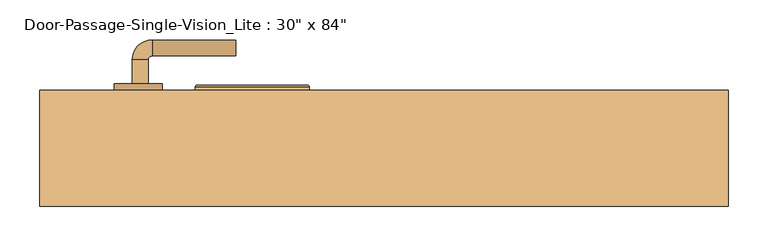
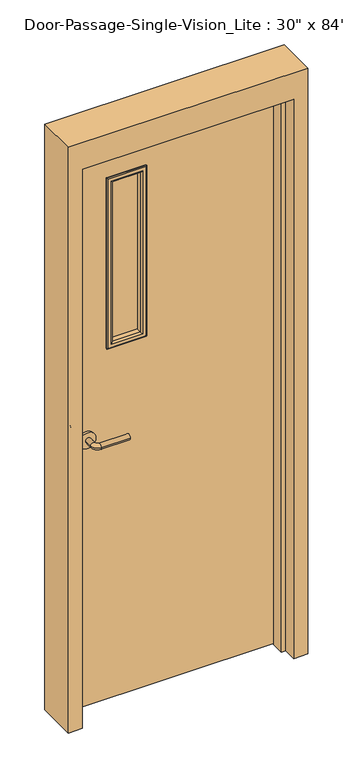
"""IFC4 building model written with IfcOpenShell, lengths in millimetres: door geometry."""

from ifc_helpers import new_model, si_unit, point, frame, frame_2d, origin, place, context, project, spatial, polyline, circle_curve, ellipse_curve, trimmed, segment, composite_curve, outline, extrude, faceted_brep, source, transform, mapped, element, save
from ifc_brep_helpers import plane_surface, cylinder_surface, revolved_surface, advanced_brep


def door_e76c17f4(model_context):
    return source(origin(), model_context, "Body", "SolidModel", [
        advanced_brep(
        [(-315.990625, 42.8, 1016.0), (-295.990625, 42.8, 1016.0), (-295.990625, 12.8, 1016.0), (-315.990625, 12.8, 1016.0), (-290.990625, 7.8, 1016.0), (-290.990625, -12.2, 1016.0), (-185.990625, -12.2, 1016.0), (-185.990625, 7.8, 1016.0)],
        [
            (0, 1, circle_curve(frame((-305.990625, 42.8, 1016.0), z_axis=(0.0, 1.0, 0.0), x_axis=(1.0, 0.0, 0.0)), 10.0)),
            (1, 0, circle_curve(frame((-305.990625, 42.8, 1016.0), z_axis=(0.0, 1.0, 0.0), x_axis=(1.0, 0.0, 0.0)), 10.0)),
            (1, 2),
            (2, 3, circle_curve(frame((-305.990625, 12.8, 1016.0), z_axis=(0.0, 1.0, 0.0), x_axis=(1.0, 0.0, 0.0)), 10.0)),
            (3, 0),
            (3, 2, circle_curve(frame((-305.990625, 12.8, 1016.0), z_axis=(0.0, 1.0, 0.0), x_axis=(1.0, 0.0, 0.0)), 10.0)),
            (4, 5, circle_curve(frame((-290.990625, -2.2, 1016.0), z_axis=(-1.0, 0.0, 0.0), x_axis=(0.0, 1.0, 0.0)), 10.0)),
            (5, 3, circle_curve(frame((-290.990625, 12.8, 1016.0), z_axis=(0.0, 0.0, -1.0), x_axis=(-1.0, 0.0, 0.0)), 25.0)),
            (2, 4, circle_curve(frame((-290.990625, 12.8, 1016.0), z_axis=(0.0, 0.0, 1.0), x_axis=(-1.0, 0.0, 0.0)), 5.0)),
            (5, 4, circle_curve(frame((-290.990625, -2.2, 1016.0), z_axis=(-1.0, 0.0, 0.0), x_axis=(0.0, 1.0, 0.0)), 10.0)),
            (6, 7, circle_curve(frame((-185.990625, -2.2, 1016.0), z_axis=(1.0, 0.0, 0.0), x_axis=(0.0, 1.0, 0.0)), 10.0)),
            (7, 6, circle_curve(frame((-185.990625, -2.2, 1016.0), z_axis=(1.0, 0.0, 0.0), x_axis=(0.0, 1.0, 0.0)), 10.0)),
            (4, 7),
            (6, 5),
        ],
        [
            plane_surface(frame((-305.990625, 42.8, 1016.0), z_axis=(0.0, 1.0, 0.0), x_axis=(0.0, 0.0, 1.0))),
            cylinder_surface(frame((-305.990625, 42.8, 1016.0), z_axis=(0.0, 1.0, 0.0), x_axis=(1.0, 0.0, 0.0)), 10.0),
            revolved_surface(trimmed(ellipse_curve(frame((-305.990625, 12.8, 1016.0), z_axis=(0.0, -1.0, 0.0), x_axis=(1.0, 0.0, 0.0)), 10.0, 10.0), [point((-315.990625, 12.8, 1016.0))], [point((-295.990625, 12.8, 1016.0))], True, "CARTESIAN"), (-290.990625, 12.8, 1016.0), (0.0, 0.0, -1.0)),
            revolved_surface(trimmed(ellipse_curve(frame((-305.990625, 12.8, 1016.0), z_axis=(0.0, -1.0, 0.0), x_axis=(1.0, 0.0, 0.0)), 10.0, 10.0), [point((-295.990625, 12.8, 1016.0))], [point((-315.990625, 12.8, 1016.0))], True, "CARTESIAN"), (-290.990625, 12.8, 1016.0), (0.0, 0.0, -1.0)),
            plane_surface(frame((-185.990625, -2.2, 1016.0), z_axis=(1.0, 0.0, 0.0), x_axis=(0.0, 0.0, 1.0))),
            cylinder_surface(frame((-290.990625, -2.2, 1016.0), z_axis=(-1.0, 0.0, 0.0), x_axis=(0.0, 1.0, 0.0)), 10.0),
        ],
        [
            (0, [[1, 2]]),
            (1, [[3, 4, 5, -2]]),
            (1, [[-5, 6, -3, -1]]),
            (2, [[7, 8, -4, 9]]),
            (3, [[10, -9, -6, -8]]),
            (4, [[11, 12]]),
            (5, [[13, -11, 14, -7]]),
            (5, [[-14, -12, -13, -10]]),
        ],
    ),
        extrude(outline(composite_curve([segment(trimmed(circle_curve(frame_2d((1016.0, -308.490625)), 30.0), [point((1016.0, -338.490625))], [point((1016.0, -278.490625))], False, "CARTESIAN"), True, "CONTINUOUS"), segment(trimmed(circle_curve(frame_2d((1016.0, -308.490625)), 30.0), [point((1016.0, -278.490625))], [point((1016.0, -338.490625))], False, "CARTESIAN"), True, "CONTINUOUS")], self_intersect=False)), frame((0.0, 42.8, 0.0), z_axis=(0.0, 1.0, 0.0), x_axis=(0.0, 0.0, 1.0)), (0.0, 0.0, 1.0), 8.0),
        advanced_brep(
        [(-315.990625, 103.25, 1016.0), (-295.990625, 103.25, 1016.0), (-315.990625, 133.25, 1016.0), (-295.990625, 133.25, 1016.0), (-290.990625, 138.25, 1016.0), (-290.990625, 158.25, 1016.0), (-185.990625, 158.25, 1016.0), (-185.990625, 138.25, 1016.0)],
        [
            (0, 1, circle_curve(frame((-305.990625, 103.25, 1016.0), z_axis=(0.0, -1.0, 0.0), x_axis=(1.0, 0.0, 0.0)), 10.0)),
            (1, 0, circle_curve(frame((-305.990625, 103.25, 1016.0), z_axis=(0.0, -1.0, 0.0), x_axis=(1.0, 0.0, 0.0)), 10.0)),
            (0, 2),
            (2, 3, circle_curve(frame((-305.990625, 133.25, 1016.0), z_axis=(0.0, -1.0, 0.0), x_axis=(1.0, 0.0, 0.0)), 10.0)),
            (3, 1),
            (3, 2, circle_curve(frame((-305.990625, 133.25, 1016.0), z_axis=(0.0, -1.0, 0.0), x_axis=(1.0, 0.0, 0.0)), 10.0)),
            (4, 3, circle_curve(frame((-290.990625, 133.25, 1016.0), z_axis=(0.0, 0.0, 1.0), x_axis=(-1.0, 0.0, 0.0)), 5.0)),
            (2, 5, circle_curve(frame((-290.990625, 133.25, 1016.0), z_axis=(0.0, 0.0, -1.0), x_axis=(-1.0, 0.0, 0.0)), 25.0)),
            (5, 4, circle_curve(frame((-290.990625, 148.25, 1016.0), z_axis=(-1.0, 0.0, 0.0), x_axis=(0.0, -1.0, 0.0)), 10.0)),
            (4, 5, circle_curve(frame((-290.990625, 148.25, 1016.0), z_axis=(-1.0, 0.0, 0.0), x_axis=(0.0, -1.0, 0.0)), 10.0)),
            (6, 7, circle_curve(frame((-185.990625, 148.25, 1016.0), z_axis=(1.0, 0.0, 0.0), x_axis=(0.0, -1.0, 0.0)), 10.0)),
            (7, 6, circle_curve(frame((-185.990625, 148.25, 1016.0), z_axis=(1.0, 0.0, 0.0), x_axis=(0.0, -1.0, 0.0)), 10.0)),
            (5, 6),
            (7, 4),
        ],
        [
            plane_surface(frame((-305.990625, 103.25, 1016.0), z_axis=(0.0, -1.0, 0.0), x_axis=(0.0, 0.0, 1.0))),
            cylinder_surface(frame((-305.990625, 103.25, 1016.0), z_axis=(0.0, -1.0, 0.0), x_axis=(1.0, 0.0, 0.0)), 10.0),
            revolved_surface(trimmed(ellipse_curve(frame((-305.990625, 133.25, 1016.0), z_axis=(0.0, -1.0, 0.0), x_axis=(1.0, 0.0, 0.0)), 10.0, 10.0), [point((-315.990625, 133.25, 1016.0))], [point((-295.990625, 133.25, 1016.0))], True, "CARTESIAN"), (-290.990625, 133.25, 1016.0), (0.0, 0.0, -1.0)),
            revolved_surface(trimmed(ellipse_curve(frame((-305.990625, 133.25, 1016.0), z_axis=(0.0, -1.0, 0.0), x_axis=(1.0, 0.0, 0.0)), 10.0, 10.0), [point((-295.990625, 133.25, 1016.0))], [point((-315.990625, 133.25, 1016.0))], True, "CARTESIAN"), (-290.990625, 133.25, 1016.0), (0.0, 0.0, -1.0)),
            plane_surface(frame((-185.990625, 148.25, 1016.0), z_axis=(1.0, 0.0, 0.0), x_axis=(0.0, 0.0, 1.0))),
            cylinder_surface(frame((-290.990625, 148.25, 1016.0), z_axis=(-1.0, 0.0, 0.0), x_axis=(0.0, -1.0, 0.0)), 10.0),
        ],
        [
            (0, [[1, 2]]),
            (1, [[-1, 3, 4, 5]]),
            (1, [[-2, -5, 6, -3]]),
            (2, [[7, -4, 8, 9]]),
            (3, [[-8, -6, -7, 10]]),
            (4, [[11, 12]]),
            (5, [[-9, 13, -12, 14]]),
            (5, [[-10, -14, -11, -13]]),
        ],
    ),
        extrude(outline(composite_curve([segment(trimmed(circle_curve(frame_2d((1016.0, -308.490625)), 30.0), [point((1016.0, -338.490625))], [point((1016.0, -278.490625))], False, "CARTESIAN"), True, "CONTINUOUS"), segment(trimmed(circle_curve(frame_2d((1016.0, -308.490625)), 30.0), [point((1016.0, -278.490625))], [point((1016.0, -338.490625))], False, "CARTESIAN"), True, "CONTINUOUS")], self_intersect=False)), frame((0.0, 95.25, 0.0), z_axis=(0.0, 1.0, 0.0), x_axis=(0.0, 0.0, 1.0)), (0.0, 0.0, 1.0), 8.0),
        faceted_brep([(381.0, 46.0375, 0.0), (381.0, 95.25, 0.0), (431.8, 95.25, 0.0), (431.8, -50.8, 0.0), (381.0, -50.8, 0.0), (381.0, -1.5875, 0.0), (365.125, -1.5875, 0.0), (365.125, 46.0375, 0.0), (381.0, 46.0375, 2133.6), (381.0, 95.25, 2133.6), (-381.0, 95.25, 2133.6), (-381.0, 95.25, 0.0), (-431.8, 95.25, 0.0), (-431.8, 95.25, 2235.2), (431.8, 95.25, 2235.2), (431.8, -50.8, 2235.2), (-431.8, -50.8, 2235.2), (-431.8, -50.8, 0.0), (-381.0, -50.8, 0.0), (-381.0, -50.8, 2133.6), (381.0, -50.8, 2133.6), (381.0, -1.5875, 2133.6), (-381.0, -1.5875, 2133.6), (-381.0, -1.5875, 0.0), (-365.125, -1.5875, 0.0), (-365.125, -1.5875, 2117.725), (365.125, -1.5875, 2117.725), (365.125, 46.0375, 2117.725), (-365.125, 46.0375, 2117.725), (-365.125, 46.0375, 0.0), (-381.0, 46.0375, 0.0), (-381.0, 46.0375, 2133.6)], [[[0, 1, 2, 3, 4, 5, 6, 7]], [[1, 0, 8, 9]], [[2, 1, 9, 10, 11, 12, 13, 14]], [[3, 2, 14, 15]], [[4, 3, 15, 16, 17, 18, 19, 20]], [[5, 4, 20, 21]], [[6, 5, 21, 22, 23, 24, 25, 26]], [[7, 6, 26, 27]], [[0, 7, 27, 28, 29, 30, 31, 8]], [[9, 8, 31, 10]], [[20, 19, 22, 21]], [[26, 25, 28, 27]], [[12, 11, 30, 29, 24, 23, 18, 17]], [[11, 10, 31, 30]], [[13, 12, 17, 16]], [[19, 18, 23, 22]], [[25, 24, 29, 28]], [[15, 14, 13, 16]]]),
        extrude(outline(polyline([(2133.6, -381.0), (0.0, -381.0), (0.0, 381.0), (2133.6, 381.0), (2133.6, -381.0)]), holes=[polyline([(1981.2, -228.6), (1981.2, -101.6), (1346.2, -101.6), (1346.2, -228.6), (1981.2, -228.6)])]), frame((0.0, 50.8, 0.0), z_axis=(0.0, 1.0, 0.0), x_axis=(0.0, 0.0, 1.0)), (0.0, 0.0, 1.0), 44.45),
        extrude(outline(polyline([(-101.6, 69.85), (-228.6, 69.85), (-228.6, 76.2), (-101.6, 76.2), (-101.6, 69.85)])), frame((0.0, 0.0, 1346.2), z_axis=(0.0, 0.0, 1.0), x_axis=(1.0, 0.0, 0.0)), (0.0, 0.0, 1.0), 635.0),
        advanced_brep(
        [(-228.6, 69.85, 1346.2), (-228.6, 50.8, 1346.2), (-228.6, 50.8, 1981.2), (-228.6, 69.85, 1981.2), (-216.6, 49.8, 1358.2), (-216.6, 69.85, 1358.2), (-216.6, 69.85, 1969.2), (-216.6, 49.8, 1969.2), (-221.6, 44.8, 1353.2), (-221.6, 44.8, 1974.2), (-236.6, 46.8, 1338.2), (-234.6, 44.8, 1340.2), (-234.6, 44.8, 1987.2), (-236.6, 46.8, 1989.2), (-236.6, 50.8, 1338.2), (-236.6, 50.8, 1989.2), (-101.6, 50.8, 1981.2), (-101.6, 69.85, 1981.2), (-113.6, 69.85, 1969.2), (-113.6, 49.8, 1969.2), (-108.6, 44.8, 1974.2), (-95.6, 44.8, 1987.2), (-93.6, 46.8, 1989.2), (-93.6, 50.8, 1989.2), (-101.6, 50.8, 1346.2), (-101.6, 69.85, 1346.2), (-113.6, 69.85, 1358.2), (-113.6, 49.8, 1358.2), (-108.6, 44.8, 1353.2), (-95.6, 44.8, 1340.2), (-93.6, 46.8, 1338.2), (-93.6, 50.8, 1338.2)],
        [
            (0, 1),
            (1, 2),
            (2, 3),
            (3, 0),
            (4, 5),
            (5, 6),
            (6, 7),
            (7, 4),
            (8, 4, ellipse_curve(frame((-221.6, 49.8, 1353.2), z_axis=(-0.7071067811865475, 0.0, 0.7071067811865475), x_axis=(-0.7071067811865474, 0.0, -0.7071067811865476)), 7.0710678, 5.0)),
            (7, 9, ellipse_curve(frame((-221.6, 49.8, 1974.2), z_axis=(-0.7071067811865475, 0.0, -0.7071067811865475), x_axis=(0.7071067811865474, 0.0, -0.7071067811865476)), 7.0710678, 5.0)),
            (9, 8),
            (10, 11, ellipse_curve(frame((-234.6, 46.8, 1340.2), z_axis=(-0.7071067811865475, 0.0, 0.7071067811865475), x_axis=(-0.7071067811865474, 0.0, -0.7071067811865476)), 2.8284271, 2.0)),
            (11, 12),
            (12, 13, ellipse_curve(frame((-234.6, 46.8, 1987.2), z_axis=(-0.7071067811865475, 0.0, -0.7071067811865475), x_axis=(0.7071067811865474, 0.0, -0.7071067811865476)), 2.8284271, 2.0)),
            (13, 10),
            (14, 10),
            (13, 15),
            (15, 14),
            (2, 16),
            (16, 17),
            (17, 3),
            (6, 18),
            (18, 19),
            (19, 7),
            (19, 20, ellipse_curve(frame((-108.6, 49.8, 1974.2), z_axis=(-0.7071067811865475, 0.0, 0.7071067811865475), x_axis=(-0.7071067811865476, 0.0, -0.7071067811865474)), 7.0710678, 5.0)),
            (20, 9),
            (12, 21),
            (21, 22, ellipse_curve(frame((-95.6, 46.8, 1987.2), z_axis=(-0.7071067811865475, 0.0, 0.7071067811865475), x_axis=(-0.7071067811865476, 0.0, -0.7071067811865474)), 2.8284271, 2.0)),
            (22, 13),
            (22, 23),
            (23, 15),
            (16, 24),
            (24, 25),
            (25, 17),
            (18, 26),
            (26, 27),
            (27, 19),
            (27, 28, ellipse_curve(frame((-108.6, 49.8, 1353.2), z_axis=(0.7071067811865475, 0.0, 0.7071067811865475), x_axis=(-0.7071067811865474, 0.0, 0.7071067811865476)), 7.0710678, 5.0)),
            (28, 20),
            (21, 29),
            (29, 30, ellipse_curve(frame((-95.6, 46.8, 1340.2), z_axis=(0.7071067811865475, 0.0, 0.7071067811865475), x_axis=(-0.7071067811865474, 0.0, 0.7071067811865476)), 2.8284271, 2.0)),
            (30, 22),
            (30, 31),
            (31, 23),
            (31, 14),
            (1, 24),
            (0, 25),
            (5, 26),
            (4, 27),
            (8, 28),
            (11, 29),
            (10, 30),
        ],
        [
            plane_surface(frame((-228.6, 50.8, 1346.2), z_axis=(-1.0, 0.0, 0.0), x_axis=(0.0, 0.0, 1.0))),
            plane_surface(frame((-216.6, 69.85, 1358.2), z_axis=(1.0, 0.0, 0.0), x_axis=(0.0, 0.0, 1.0))),
            cylinder_surface(frame((-221.6, 49.8, 1346.2), z_axis=(0.0, 0.0, -1.0), x_axis=(-1.0, 0.0, 0.0)), 5.0),
            cylinder_surface(frame((-234.6, 46.8, 1346.2), z_axis=(0.0, 0.0, -1.0), x_axis=(-1.0, 0.0, 0.0)), 2.0),
            plane_surface(frame((-236.6, 46.8, 1338.2), z_axis=(-1.0, 0.0, 0.0), x_axis=(0.0, 0.0, 1.0))),
            plane_surface(frame((-228.6, 50.8, 1981.2), z_axis=(0.0, 0.0, 1.0), x_axis=(1.0, 0.0, 0.0))),
            plane_surface(frame((-216.6, 69.85, 1969.2), z_axis=(0.0, 0.0, -1.0), x_axis=(1.0, 0.0, 0.0))),
            cylinder_surface(frame((-228.6, 49.8, 1974.2), z_axis=(-1.0, 0.0, 0.0), x_axis=(0.0, 0.0, 1.0)), 5.0),
            cylinder_surface(frame((-228.6, 46.8, 1987.2), z_axis=(-1.0, 0.0, 0.0), x_axis=(0.0, 0.0, 1.0)), 2.0),
            plane_surface(frame((-236.6, 46.8, 1989.2), z_axis=(0.0, 0.0, 1.0), x_axis=(1.0, 0.0, 0.0))),
            plane_surface(frame((-101.6, 50.8, 1981.2), z_axis=(1.0, 0.0, 0.0), x_axis=(0.0, 0.0, -1.0))),
            plane_surface(frame((-113.6, 69.85, 1969.2), z_axis=(-1.0, 0.0, 0.0), x_axis=(0.0, 0.0, -1.0))),
            cylinder_surface(frame((-108.6, 49.8, 1981.2), z_axis=(0.0, 0.0, 1.0), x_axis=(1.0, 0.0, 0.0)), 5.0),
            cylinder_surface(frame((-95.6, 46.8, 1981.2), z_axis=(0.0, 0.0, 1.0), x_axis=(1.0, 0.0, 0.0)), 2.0),
            plane_surface(frame((-93.6, 46.8, 1989.2), z_axis=(1.0, 0.0, 0.0), x_axis=(0.0, 0.0, -1.0))),
            plane_surface(frame((-93.6, 50.8, 1338.2), z_axis=(0.0, 1.0, 0.0), x_axis=(-1.0, 0.0, 0.0))),
            plane_surface(frame((-101.6, 50.8, 1346.2), z_axis=(0.0, 0.0, -1.0), x_axis=(-1.0, 0.0, 0.0))),
            plane_surface(frame((-101.6, 69.85, 1346.2), z_axis=(0.0, 1.0, 0.0), x_axis=(-1.0, 0.0, 0.0))),
            plane_surface(frame((-113.6, 69.85, 1358.2), z_axis=(0.0, 0.0, 1.0), x_axis=(-1.0, 0.0, 0.0))),
            cylinder_surface(frame((-101.6, 49.8, 1353.2), z_axis=(1.0, 0.0, 0.0), x_axis=(0.0, 0.0, -1.0)), 5.0),
            plane_surface(frame((-108.6, 44.8, 1353.2), z_axis=(0.0, -1.0, 0.0), x_axis=(-1.0, 0.0, 0.0))),
            cylinder_surface(frame((-101.6, 46.8, 1340.2), z_axis=(1.0, 0.0, 0.0), x_axis=(0.0, 0.0, -1.0)), 2.0),
            plane_surface(frame((-93.6, 46.8, 1338.2), z_axis=(0.0, 0.0, -1.0), x_axis=(-1.0, 0.0, 0.0))),
        ],
        [
            (0, [[1, 2, 3, 4]]),
            (1, [[5, 6, 7, 8]]),
            (2, [[9, -8, 10, 11]]),
            (3, [[12, 13, 14, 15]]),
            (4, [[16, -15, 17, 18]]),
            (5, [[-3, 19, 20, 21]]),
            (6, [[-7, 22, 23, 24]]),
            (7, [[-10, -24, 25, 26]]),
            (8, [[-14, 27, 28, 29]]),
            (9, [[-17, -29, 30, 31]]),
            (10, [[-20, 32, 33, 34]]),
            (11, [[-23, 35, 36, 37]]),
            (12, [[-25, -37, 38, 39]]),
            (13, [[-28, 40, 41, 42]]),
            (14, [[-30, -42, 43, 44]]),
            (15, [[-31, -44, 45, -18], [46, -32, -19, -2]]),
            (16, [[-33, -46, -1, 47]]),
            (17, [[-21, -34, -47, -4], [48, -35, -22, -6]]),
            (18, [[-36, -48, -5, 49]]),
            (19, [[-38, -49, -9, 50]]),
            (20, [[51, -40, -27, -13], [-26, -39, -50, -11]]),
            (21, [[-41, -51, -12, 52]]),
            (22, [[-43, -52, -16, -45]]),
        ],
    ),
        advanced_brep(
        [(-228.6, 76.2, 1981.2), (-228.6, 95.25, 1981.2), (-228.6, 95.25, 1346.2), (-228.6, 76.2, 1346.2), (-216.6, 96.25, 1969.2), (-216.6, 76.2, 1969.2), (-216.6, 76.2, 1358.2), (-216.6, 96.25, 1358.2), (-221.6, 101.25, 1974.2), (-221.6, 101.25, 1353.2), (-236.6, 99.25, 1989.2), (-234.6, 101.25, 1987.2), (-234.6, 101.25, 1340.2), (-236.6, 99.25, 1338.2), (-236.6, 95.25, 1989.2), (-236.6, 95.25, 1338.2), (-101.6, 95.25, 1346.2), (-101.6, 76.2, 1346.2), (-113.6, 76.2, 1358.2), (-113.6, 96.25, 1358.2), (-108.6, 101.25, 1353.2), (-95.6, 101.25, 1340.2), (-93.6, 99.25, 1338.2), (-93.6, 95.25, 1338.2), (-101.6, 95.25, 1981.2), (-101.6, 76.2, 1981.2), (-113.6, 76.2, 1969.2), (-113.6, 96.25, 1969.2), (-108.6, 101.25, 1974.2), (-95.6, 101.25, 1987.2), (-93.6, 99.25, 1989.2), (-93.6, 95.25, 1989.2)],
        [
            (0, 1),
            (1, 2),
            (2, 3),
            (3, 0),
            (4, 5),
            (5, 6),
            (6, 7),
            (7, 4),
            (8, 4, ellipse_curve(frame((-221.6, 96.25, 1974.2), z_axis=(-0.7071067811865475, 0.0, -0.7071067811865475), x_axis=(-0.7071067811865474, 0.0, 0.7071067811865476)), 7.0710678, 5.0)),
            (7, 9, ellipse_curve(frame((-221.6, 96.25, 1353.2), z_axis=(-0.7071067811865475, 0.0, 0.7071067811865475), x_axis=(0.7071067811865474, 0.0, 0.7071067811865476)), 7.0710678, 5.0)),
            (9, 8),
            (10, 11, ellipse_curve(frame((-234.6, 99.25, 1987.2), z_axis=(-0.7071067811865475, 0.0, -0.7071067811865475), x_axis=(-0.7071067811865474, 0.0, 0.7071067811865476)), 2.8284271, 2.0)),
            (11, 12),
            (12, 13, ellipse_curve(frame((-234.6, 99.25, 1340.2), z_axis=(-0.7071067811865475, 0.0, 0.7071067811865475), x_axis=(0.7071067811865474, 0.0, 0.7071067811865476)), 2.8284271, 2.0)),
            (13, 10),
            (14, 10),
            (13, 15),
            (15, 14),
            (2, 16),
            (16, 17),
            (17, 3),
            (6, 18),
            (18, 19),
            (19, 7),
            (19, 20, ellipse_curve(frame((-108.6, 96.25, 1353.2), z_axis=(-0.7071067811865475, 0.0, -0.7071067811865475), x_axis=(-0.7071067811865476, 0.0, 0.7071067811865474)), 7.0710678, 5.0)),
            (20, 9),
            (12, 21),
            (21, 22, ellipse_curve(frame((-95.6, 99.25, 1340.2), z_axis=(-0.7071067811865475, 0.0, -0.7071067811865475), x_axis=(-0.7071067811865476, 0.0, 0.7071067811865474)), 2.8284271, 2.0)),
            (22, 13),
            (22, 23),
            (23, 15),
            (16, 24),
            (24, 25),
            (25, 17),
            (18, 26),
            (26, 27),
            (27, 19),
            (27, 28, ellipse_curve(frame((-108.6, 96.25, 1974.2), z_axis=(0.7071067811865475, 0.0, -0.7071067811865475), x_axis=(-0.7071067811865474, 0.0, -0.7071067811865476)), 7.0710678, 5.0)),
            (28, 20),
            (21, 29),
            (29, 30, ellipse_curve(frame((-95.6, 99.25, 1987.2), z_axis=(0.7071067811865475, 0.0, -0.7071067811865475), x_axis=(-0.7071067811865474, 0.0, -0.7071067811865476)), 2.8284271, 2.0)),
            (30, 22),
            (30, 31),
            (31, 23),
            (31, 14),
            (1, 24),
            (0, 25),
            (5, 26),
            (4, 27),
            (8, 28),
            (11, 29),
            (10, 30),
        ],
        [
            plane_surface(frame((-228.6, 95.25, 1981.2), z_axis=(-1.0, 0.0, 0.0), x_axis=(0.0, 0.0, -1.0))),
            plane_surface(frame((-216.6, 76.2, 1969.2), z_axis=(1.0, 0.0, 0.0), x_axis=(0.0, 0.0, -1.0))),
            cylinder_surface(frame((-221.6, 96.25, 1981.2), z_axis=(0.0, 0.0, 1.0), x_axis=(-1.0, 0.0, 0.0)), 5.0),
            cylinder_surface(frame((-234.6, 99.25, 1981.2), z_axis=(0.0, 0.0, 1.0), x_axis=(-1.0, 0.0, 0.0)), 2.0),
            plane_surface(frame((-236.6, 99.25, 1989.2), z_axis=(-1.0, 0.0, 0.0), x_axis=(0.0, 0.0, -1.0))),
            plane_surface(frame((-228.6, 95.25, 1346.2), z_axis=(0.0, 0.0, -1.0), x_axis=(1.0, 0.0, 0.0))),
            plane_surface(frame((-216.6, 76.2, 1358.2), z_axis=(0.0, 0.0, 1.0), x_axis=(1.0, 0.0, 0.0))),
            cylinder_surface(frame((-228.6, 96.25, 1353.2), z_axis=(-1.0, 0.0, 0.0), x_axis=(0.0, 0.0, -1.0)), 5.0),
            cylinder_surface(frame((-228.6, 99.25, 1340.2), z_axis=(-1.0, 0.0, 0.0), x_axis=(0.0, 0.0, -1.0)), 2.0),
            plane_surface(frame((-236.6, 99.25, 1338.2), z_axis=(0.0, 0.0, -1.0), x_axis=(1.0, 0.0, 0.0))),
            plane_surface(frame((-101.6, 95.25, 1346.2), z_axis=(1.0, 0.0, 0.0), x_axis=(0.0, 0.0, 1.0))),
            plane_surface(frame((-113.6, 76.2, 1358.2), z_axis=(-1.0, 0.0, 0.0), x_axis=(0.0, 0.0, 1.0))),
            cylinder_surface(frame((-108.6, 96.25, 1346.2), z_axis=(0.0, 0.0, -1.0), x_axis=(1.0, 0.0, 0.0)), 5.0),
            cylinder_surface(frame((-95.6, 99.25, 1346.2), z_axis=(0.0, 0.0, -1.0), x_axis=(1.0, 0.0, 0.0)), 2.0),
            plane_surface(frame((-93.6, 99.25, 1338.2), z_axis=(1.0, 0.0, 0.0), x_axis=(0.0, 0.0, 1.0))),
            plane_surface(frame((-93.6, 95.25, 1989.2), z_axis=(0.0, -1.0, 0.0), x_axis=(-1.0, 0.0, 0.0))),
            plane_surface(frame((-101.6, 95.25, 1981.2), z_axis=(0.0, 0.0, 1.0), x_axis=(-1.0, 0.0, 0.0))),
            plane_surface(frame((-101.6, 76.2, 1981.2), z_axis=(0.0, -1.0, 0.0), x_axis=(-1.0, 0.0, 0.0))),
            plane_surface(frame((-113.6, 76.2, 1969.2), z_axis=(0.0, 0.0, -1.0), x_axis=(-1.0, 0.0, 0.0))),
            cylinder_surface(frame((-101.6, 96.25, 1974.2), z_axis=(1.0, 0.0, 0.0), x_axis=(0.0, 0.0, 1.0)), 5.0),
            plane_surface(frame((-108.6, 101.25, 1974.2), z_axis=(0.0, 1.0, 0.0), x_axis=(-1.0, 0.0, 0.0))),
            cylinder_surface(frame((-101.6, 99.25, 1987.2), z_axis=(1.0, 0.0, 0.0), x_axis=(0.0, 0.0, 1.0)), 2.0),
            plane_surface(frame((-93.6, 99.25, 1989.2), z_axis=(0.0, 0.0, 1.0), x_axis=(-1.0, 0.0, 0.0))),
        ],
        [
            (0, [[1, 2, 3, 4]]),
            (1, [[5, 6, 7, 8]]),
            (2, [[9, -8, 10, 11]]),
            (3, [[12, 13, 14, 15]]),
            (4, [[16, -15, 17, 18]]),
            (5, [[-3, 19, 20, 21]]),
            (6, [[-7, 22, 23, 24]]),
            (7, [[-10, -24, 25, 26]]),
            (8, [[-14, 27, 28, 29]]),
            (9, [[-17, -29, 30, 31]]),
            (10, [[-20, 32, 33, 34]]),
            (11, [[-23, 35, 36, 37]]),
            (12, [[-25, -37, 38, 39]]),
            (13, [[-28, 40, 41, 42]]),
            (14, [[-30, -42, 43, 44]]),
            (15, [[-31, -44, 45, -18], [46, -32, -19, -2]]),
            (16, [[-33, -46, -1, 47]]),
            (17, [[-21, -34, -47, -4], [48, -35, -22, -6]]),
            (18, [[-36, -48, -5, 49]]),
            (19, [[-38, -49, -9, 50]]),
            (20, [[51, -40, -27, -13], [-26, -39, -50, -11]]),
            (21, [[-41, -51, -12, 52]]),
            (22, [[-43, -52, -16, -45]]),
        ],
    ),
    ])


if __name__ == "__main__":
    model = new_model("IFC4")
    model_context = context("Model", 3, world=origin())
    ifc_project = project(units=[si_unit("LENGTHUNIT", "METRE", prefix="MILLI")], contexts=[model_context])
    site = spatial("IfcSite", under=ifc_project)
    building = spatial("IfcBuilding", under=site)
    placement = place(None, origin())
    door_shape = door_e76c17f4(model_context)
    element("IfcDoor", 1, ObjectType="Door-Passage-Single-Vision_Lite : 30\" x 84\"", at=placement, inside=building, context=model_context, shape_type="MappedRepresentation", body=[
        mapped(door_shape, transform((0.0, 0.0, 0.0), x_axis=(1.0, 0.0, 0.0), y_axis=(0.0, 1.0, 0.0), z_axis=(0.0, 0.0, 1.0))),
    ])
    save(model, "model.ifc")

# Revit data of these elements
# Type "Door-Passage-Single-Vision_Lite : 30\" x 84\""
#   Type Mark = "20"
#   Assembly Code = "B2030100"
#   Analytic Construction = "Wooden"
#   Thickness = 0' - 1 3/4"
#   Thermal Resistance (R) = 2.5876 (h·ft²·°F)/BTU
#   Swing Angle [instance default] = 90.00°
#   Strike Height = 3' - 4"
#   Rough Width [instance default] = 2' - 10"
#   Rough Height [instance default] = 7' - 4"
#   MFOpeningHeight [instance default] = 0' - 4"
#   MFOpeningWidth [instance default] = 0' - 4"
#   Inset Calculate [instance default] = 0' - 4"
#   Masonry Inset [instance default] = 0' - 1"
#   Height = 7' - 0"
#   Width = 2' - 6"
#   Heat Transfer Coefficient (U) = 0.3865 BTU/(h·ft²·°F)
#   Masonry Frame Depth = 0' - 5 3/4"
#   Masonry Frame [instance default] = yes
#   Function = 1
#   Dry Wall Frame [instance default] = no
#   Define Thermal Properties by = 1
#   Panel Material = Wood - Birch
#   Glazing = Glass
#   Glass Stop Material = Metal - Paint Finish - Grey
#   Frame Material = Metal - Paint Finish - Grey
#   Door Handle Material = Aluminum
#   Visual Light Transmittance = 0
#   Solar Heat Gain Coefficient = 0
#   Wall Closure = (empty or 0)
# Element 1 (IfcDoor, "Door-Passage-Single-Vision_Lite : 30\" x 84\"")
#   Materials on its faces: "Metal - Paint Finish - Grey", "Aluminum", "Wood - Birch", "Glass"
# Materials
#   "Wood - Birch": class "Wood", colour RGB 173 132 96, transparency 0, Cost = 0
#   "Glass": class "Glass", colour RGB 245 245 243, transparency 1, Description = "Soda Lime Glass", Cost = 0
#   "Metal - Paint Finish - Grey": class "Paint", colour RGB 178 178 178, transparency 0, Cost = 0
#   "Aluminum": class "Metal", colour RGB 244 245 246, transparency 0, Description = "Aluminum 6061", Cost = 0
